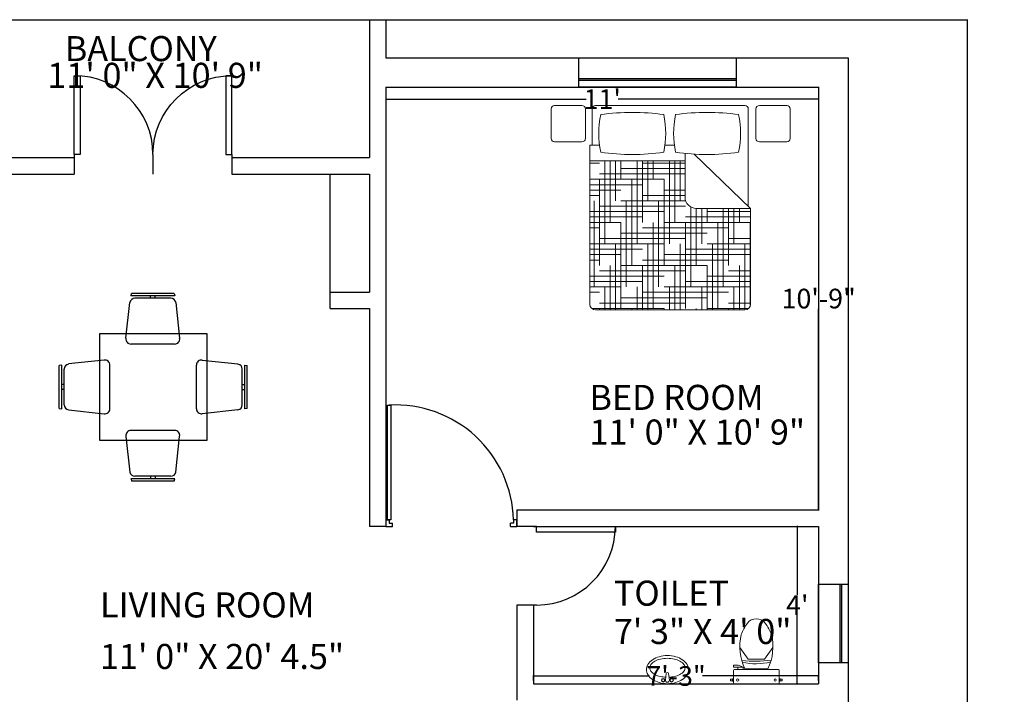
# Model space of a CAD drawing. Units: inches. Extents: x -113 to 5399, y -1393 to 3302.
# Tile 30 of 40: x 3870 to 4170, y 356 to 561. Entities that reach past the tile are written whole.
import ezdxf

# ---------------------------------------------------------------- set-up
doc = ezdxf.new("R2010")
doc.units = ezdxf.units.IN
doc.header["$MEASUREMENT"] = 0
for name, color, linetype, lineweight in [('A-ANNO-DIMS', 254, 'Continuous', 18), ('A-AREA-IDEN', 4, 'Continuous', 18), ('A-FLOR-FIXT', 8, 'Continuous', 18), ('doors', 2, 'Continuous', 25), ('furniture', 131, 'Continuous', 18), ('walls', 1, 'Continuous', 25), ('windows', 3, 'Continuous', 25)]:
    doc.layers.add(name, color=color, linetype=linetype, lineweight=lineweight)
doc.layers.add('B-FURNITURE', color=22, linetype='Continuous')
doc.styles.get("Standard").update_dxf_attribs({"font": 'arial.ttf'})
doc.dimstyles.get("Standard").update_dxf_attribs({"dimtxt": 6, "dimasz": 0.18, "dimexe": 0.18, "dimexo": 0.0625, "dimgap": 0.09, "dimtad": 0, "dimtih": 1, "dimtoh": 1, "dimdec": 1, "dimzin": 0, "dimdsep": 46, "dimlunit": 4, "dimtxsty": 'Standard', "dimblk": 'ARCHTICK', "dimcen": 0.09, "dimadec": 0, "dimazin": 0, "dimtfac": 1, "dimtdec": 1, "dimtofl": 0, "dimtmove": 0, "dimatfit": 3, "dimfxl": 1, "dimtolj": 1, "dimtzin": 0, "dimarcsym": 0})

# ---------------------------------------------------------------- blocks, each defined once
blk = doc.blocks.new('*U2')
for p, q in [((0, 0), (0, -6)), ((24, 0), (24, -6))]:
    blk.add_line(p, q)
blk.add_lwpolyline([(0, 0), (0, 24), (1.75, 24), (1.75, 0)], close=True)
blk.add_arc((0, 0), 24, 0, 90)
blk = doc.blocks.new('*X4')
at = {"color": 0}
for p, q in [((4.3594, 18.5625), (4.3594, 18.6457)), ((4.5, 18), (4.5, 18.6457)), ((4.5469, 18.1875), (4.5469, 18.6457)), ((4.5938, 18.375), (4.5938, 18.6457)), ((4.6406, 18.5625), (4.6406, 18.6457)), ((4.6875, 18.6094), (5.4375, 18.6094)), ((4.7812, 18), (4.7812, 18.6457)), ((4.8281, 18.1875), (4.8281, 18.6457)), ((4.875, 18.375), (4.875, 18.6457)), ((4.9219, 18.5625), (4.9219, 18.6457)), ((5.0625, 18), (5.0625, 18.6457)), ((5.1094, 18.1875), (5.1094, 18.6457)), ((5.1562, 18.375), (5.1562, 18.6457)), ((5.2031, 18.5625), (5.2031, 18.6457)), ((5.3438, 18), (5.3438, 18.6457)), ((5.3906, 18.1875), (5.3906, 18.6457)), ((5.4375, 18.375), (5.4375, 18.6457)), ((5.4844, 18.5625), (5.4844, 18.6457)), ((5.625, 18), (5.625, 18.6287)), ((4.4531, 17.8169), (4.4531, 18.5625)), ((4.5, 18.5625), (5.25, 18.5625)), ((4.7344, 17.8125), (4.7344, 18.5625)), ((5.0156, 17.8125), (5.0156, 18.5625)), ((5.2969, 17.8125), (5.2969, 18.5625)), ((5.5781, 17.8125), (5.5781, 18.5625)), ((5.625, 18.5625), (5.6375, 18.5625)), ((4.3395, 18.5156), (5.0625, 18.5156)), ((4.3395, 18.4688), (4.875, 18.4688)), ((5.25, 18.4688), (5.6375, 18.4688)), ((5.4375, 18.5156), (5.6375, 18.5156)), ((4.3395, 18.4219), (4.6875, 18.4219)), ((4.3395, 18.375), (4.5, 18.375)), ((4.4062, 17.8169), (4.4062, 18.375)), ((4.6875, 17.8114), (4.6875, 18.375)), ((4.875, 18.375), (5.625, 18.375)), ((4.9688, 17.625), (4.9688, 18.375)), ((5.0625, 18.4219), (5.6375, 18.4219)), ((5.25, 17.625), (5.25, 18.375)), ((5.5312, 17.625), (5.5312, 18.375)), ((4.5, 18.2812), (5.25, 18.2812)), ((4.6875, 18.3281), (5.4375, 18.3281)), ((5.625, 18.2812), (5.6375, 18.2812)), ((4.3395, 18.2344), (5.0625, 18.2344)), ((4.3395, 18.1875), (4.875, 18.1875)), ((4.3594, 17.8169), (4.3594, 18.1875)), ((4.6406, 17.8169), (4.6406, 18.1875)), ((4.9219, 17.4375), (4.9219, 18.1875)), ((5.2031, 17.4375), (5.2031, 18.1875)), ((5.25, 18.1875), (5.6375, 18.1875)), ((5.4375, 18.2344), (5.6375, 18.2344)), ((5.4844, 17.4375), (5.4844, 18.1875)), ((4.3395, 18.1406), (4.6875, 18.1406)), ((4.3395, 18.0938), (4.5, 18.0938)), ((4.875, 18.0938), (5.625, 18.0938)), ((5.0625, 18.1406), (5.6375, 18.1406)), ((4.6875, 18.0469), (5.4375, 18.0469)), ((4.3395, 17.9531), (5.0625, 17.9531)), ((4.5, 18), (5.25, 18)), ((4.5938, 17.8169), (4.5938, 18)), ((4.875, 17.25), (4.875, 18)), ((5.1562, 17.25), (5.1562, 18)), ((5.4375, 17.25), (5.4375, 18)), ((5.4375, 17.9531), (5.6375, 17.9531)), ((5.625, 18), (5.6375, 18)), ((4.3395, 17.9062), (4.875, 17.9062)), ((4.3395, 17.8594), (4.6875, 17.8594)), ((5.0625, 17.8594), (5.6375, 17.8594)), ((5.25, 17.9062), (5.6375, 17.9062)), ((4.7421, 17.7656), (5.4375, 17.7656)), ((4.8281, 17.2457), (4.8281, 17.8125)), ((4.875, 17.8125), (5.625, 17.8125)), ((5.1094, 17.2457), (5.1094, 17.8125)), ((5.3906, 17.2457), (5.3906, 17.8125)), ((4.7548, 17.7188), (5.25, 17.7188)), ((4.7548, 17.6719), (5.0625, 17.6719)), ((5.4375, 17.6719), (5.6375, 17.6719)), ((5.625, 17.7188), (5.6375, 17.7188)), ((4.7548, 17.625), (4.875, 17.625)), ((4.7812, 17.2457), (4.7812, 17.625)), ((5.0625, 17.2457), (5.0625, 17.625)), ((5.0625, 17.5781), (5.6375, 17.5781)), ((5.25, 17.625), (5.6375, 17.625)), ((5.3438, 17.2457), (5.3438, 17.625)), ((5.625, 17.2627), (5.625, 17.625)), ((4.875, 17.5312), (5.625, 17.5312)), ((4.7548, 17.4844), (5.4375, 17.4844)), ((4.7548, 17.4375), (5.25, 17.4375)), ((5.0156, 17.2457), (5.0156, 17.4375)), ((5.2969, 17.2457), (5.2969, 17.4375)), ((5.5781, 17.2457), (5.5781, 17.4375)), ((5.625, 17.4375), (5.6375, 17.4375)), ((4.7548, 17.3906), (5.0625, 17.3906)), ((4.7548, 17.3438), (4.875, 17.3438)), ((5.25, 17.3438), (5.6375, 17.3438)), ((5.4375, 17.3906), (5.6375, 17.3906)), ((4.875, 17.25), (5.6077, 17.25)), ((4.9688, 17.2457), (4.9688, 17.25)), ((5.0625, 17.2969), (5.6375, 17.2969)), ((5.25, 17.2457), (5.25, 17.25)), ((5.5312, 17.2457), (5.5312, 17.25))]:
    blk.add_line(p, q, dxfattribs=at)
blk = doc.blocks.new('MAT-P01')
for p, q in [((-0.0213, 0.8164), (-0.0213, 0.5605)), ((0.0087, 0.8464), (0.2471, 0.8464)), ((0.2771, 0.8164), (0.2771, 0.5605)), ((0.3437, 0.8164), (0.3437, -0.0316)), ((0.3737, 0.8464), (1.6737, 0.8464)), ((1.7037, 0.8164), (1.7037, 0.5005)), ((1.7622, 0.8164), (1.7622, 0.5605)), ((1.7922, 0.8464), (2.0306, 0.8464)), ((2.0606, 0.8164), (2.0606, 0.5605)), ((0.0087, 0.5305), (0.2471, 0.5305)), ((1.7922, 0.5305), (2.0306, 0.5305)), ((0.8949, 0.4293), (0.8949, 0.0491)), ((0.9879, 0.5005), (1.0693, 0.5005)), ((1.6393, 0.5005), (1.7237, 0.5005)), ((1.7237, 0.5005), (1.7237, -0.8836)), ((0.8146, 0.423), (0.3237, -0.0509)), ((0.8949, 0.3643), (1.7237, 0.3643)), ((0.8949, 0.3643), (0.8949, 0.0491)), ((0.8949, 0.3643), (1.7237, 0.3643)), ((1.7237, 0.3643), (1.7237, -0.8836)), ((0.3237, -0.0509), (0.7949, -0.0509)), ((0.3237, -0.0509), (0.3237, -0.8836)), ((0.3737, -0.9336), (1.6737, -0.9336))]:
    blk.add_line(p, q)
for centre, radius, start, end in [((0.0087, 0.8164), 0.03, 90, 180), ((0.2471, 0.8164), 0.03, 0, 90), ((0.3737, 0.8164), 0.03, 90, 180), ((0.7029, -1.1436), 1.9306, 81.81622, 98.18378), ((1.3543, -1.1436), 1.9306, 81.81622, 98.18378), ((1.6737, 0.8164), 0.03, 0, 90), ((1.7922, 0.8164), 0.03, 90, 180), ((2.0306, 0.8164), 0.03, 0, 90), ((1.2251, 0.6034), 0.8138, 168.37298, 191.62702), ((0.1806, 0.6034), 0.8138, 348.37298, 11.62702), ((1.8766, 0.6034), 0.8138, 168.37298, 191.62702), ((0.8321, 0.6034), 0.8138, 348.37298, 11.62702), ((0.0087, 0.5605), 0.03, 180, 270), ((0.2471, 0.5605), 0.03, 270, 0), ((1.7922, 0.5605), 0.03, 180, 270), ((2.0306, 0.5605), 0.03, 270, 0), ((0.7029, 2.3504), 1.9306, 261.81622, 278.18378), ((1.3543, 2.3504), 1.9306, 261.81622, 278.18378), ((0.7949, 0.0491), 0.1, 270, 0), ((0.3737, -0.8836), 0.05, 180, 270), ((1.6737, -0.8836), 0.05, 270, 0)]:
    blk.add_arc(centre, radius, start, end)
at = {"rotation": 270}
blk.add_blockref('*X4', (-16.9221, 4.7038), dxfattribs=at)
blk = doc.blocks.new('A$C6ACA79D1')
at = {"layer": 'B-FURNITURE'}
for p, q in [((-0.5034, 0.0535), (-0.8012, -0.2442)), ((-0.4835, 0.0392), (-0.7869, -0.2642)), ((-0.5034, 0.0535), (-0.4835, 0.0392)), ((-0.4291, 0.0003), (-0.1547, -0.2204)), ((0.7869, -0.259), (0.4835, 0.0444)), ((0.4842, 0.0434), (0.5041, 0.0577)), ((0.7427, -0.249), (0.4935, 0.0002)), ((0.8012, -0.239), (0.5034, 0.0587)), ((-0.4935, -0.005), (-0.7427, -0.2542)), ((-0.601, -0.1125), (-0.6181, -0.0954)), ((0.601, -0.1073), (0.6181, -0.0902)), ((-0.6352, -0.1467), (-0.6523, -0.1296)), ((0.6352, -0.1415), (0.6523, -0.1244)), ((-0.7859, -0.2635), (-0.8002, -0.2436)), ((0.8012, -0.239), (0.7869, -0.259)), ((-0.1485, -0.2964), (-0.4513, -0.5992)), ((0.4513, -0.594), (0.1485, -0.2912)), ((0.748, -0.3133), (0.5273, -0.5877)), ((-0.1485, -1.1937), (-0.4513, -0.8909)), ((0.4513, -0.8961), (0.1485, -1.199)), ((0.748, -1.1768), (0.5273, -0.9024)), ((-0.5034, -1.5436), (-0.8012, -1.2459)), ((-0.7859, -1.2266), (-0.8002, -1.2466)), ((-0.4835, -1.5293), (-0.7869, -1.226)), ((-0.4935, -1.4851), (-0.7427, -1.236)), ((0.7869, -1.2312), (0.4835, -1.5346)), ((0.7427, -1.2412), (0.4935, -1.4903)), ((0.8012, -1.2511), (0.5034, -1.5488)), ((0.8012, -1.2511), (0.7869, -1.2312)), ((-0.6352, -1.3434), (-0.6523, -1.3605)), ((-0.4291, -1.4904), (-0.1547, -1.2698)), ((0.6352, -1.3486), (0.6523, -1.3657)), ((-0.601, -1.3776), (-0.6181, -1.3948)), ((0.601, -1.3829), (0.6181, -1.4)), ((-0.5034, -1.5436), (-0.4835, -1.5293)), ((0.4842, -1.5336), (0.5041, -1.5478))]:
    blk.add_line(p, q, dxfattribs=at)
at = {"layer": 'B-FURNITURE', "ltscale": 300}
for p, q in [((0.1547, -0.2152), (0.4291, 0.0055)), ((-0.5273, -0.593), (-0.748, -0.3186)), ((-0.5273, -0.8972), (-0.748, -1.1716)), ((0.1547, -1.275), (0.4291, -1.4956))]:
    blk.add_line(p, q, dxfattribs=at)
blk.add_lwpolyline([(-0.7425, -0.7425), (0, 0), (0.7425, -0.7425), (0, -1.4849)], close=True, dxfattribs=at)
at = {"layer": 'B-FURNITURE', "ltscale": 400}
for centre, start, end in [((-0.4582, -0.0403), 54.40695, 135), ((0.4589, -0.0361), 45, 125.59305), ((-0.7063, -0.2888), 135, 215.59305), ((0.7073, -0.2843), 324.40695, 45), ((-0.7063, -1.2013), 144.40695, 225), ((0.7073, -1.2059), 315, 35.59305), ((-0.4582, -1.4498), 225, 305.59305), ((0.4589, -1.454), 234.40695, 315)]:
    blk.add_arc(centre, 0.0499, start, end, dxfattribs=at)
at = {"layer": 'B-FURNITURE', "ltscale": 300}
for centre, start, end in [((-0.1838, -0.261), 315, 54.40695), ((0.1838, -0.2558), 125.59305, 225), ((-0.4866, -0.5639), 215.59305, 315), ((0.4866, -0.5586), 225, 324.40695), ((-0.4866, -0.9263), 45, 144.40695), ((0.4866, -0.9315), 35.59305, 135), ((-0.1838, -1.2291), 305.59305, 45), ((0.1838, -1.2343), 135, 234.40695)]:
    blk.add_arc(centre, 0.05, start, end, dxfattribs=at)
blk = doc.blocks.new('toilet-3')
at = {"color": 0, "linetype": 'ByBlock'}
for p, q in [((-0.281, -0.05), (-0.281, -0.069)), ((-0.281, -0.05), (-0.261, -0.05)), ((-0.281, -0.069), (-0.261, -0.069)), ((-0.261, -0.047), (-0.261, -0.072)), ((-0.261, -0.047), (-0.251, -0.047)), ((-0.261, -0.072), (-0.251, -0.072)), ((-0.251, -0.047), (-0.251, -0.072)), ((-0.25, -0.03), (-0.25, -0.165)), ((0.24, -0.02), (-0.24, -0.02)), ((0.25, -0.03), (0.25, -0.165)), ((0.261, -0.047), (0.251, -0.047)), ((0.251, -0.047), (0.251, -0.072)), ((0.261, -0.072), (0.251, -0.072)), ((0.261, -0.047), (0.261, -0.072)), ((0.281, -0.05), (0.261, -0.05)), ((0.281, -0.069), (0.261, -0.069)), ((0.281, -0.05), (0.281, -0.069)), ((-0.144, -0.2), (-0.25, -0.2)), ((-0.25, -0.2), (-0.25, -0.222)), ((0.24, -0.175), (-0.24, -0.175)), ((-0.202, -0.2), (-0.202, -0.175)), ((-0.198, -0.222), (-0.16, -0.207)), ((-0.16, -0.207), (-0.16, -0.2)), ((-0.144, -0.2), (-0.144, -0.175)), ((0.125, -0.182), (-0.125, -0.182)), ((-0.198, -0.222), (-0.25, -0.222)), ((-0.089, -0.287), (-0.18, -0.415)), ((0.089, -0.287), (-0.089, -0.287)), ((0.089, -0.287), (0.18, -0.415))]:
    blk.add_line(p, q, dxfattribs=at)
for centre in [(-0.205, -0.059), (0.205, -0.059)]:
    blk.add_circle(centre, 0.0125, dxfattribs=at)
for centre, radius, start, end in [((-0.24, -0.03), 0.01, 90, 180), ((0.24, -0.03), 0.01, 0, 90), ((-0.24, -0.165), 0.01, 180, 270), ((0.376, -0.424), 0.557, 154.2321, 193.6755), ((-0.376, -0.424), 0.557, 346.3245, 25.7679), ((0.24, -0.165), 0.01, 270, 0), ((-0.013, -1.787), 1.521, 83.4552, 95.5271), ((-0.005, -0.896), 0.659, 75.9276, 103.0204), ((0.262, -0.406), 0.452, 199.2942, 217.2549), ((-0.265, -0.4), 0.457, 322.2382, 340.1051), ((-0.001, -0.609), 0.12, 216.3794, 323.6206)]:
    blk.add_arc(centre, radius, start, end, dxfattribs=at)
blk = doc.blocks.new('wash-6')
at = {"color": 0, "linetype": 'ByBlock'}
for p, q in [((-0.036, -0.063), (-0.021, -0.18)), ((0.036, -0.063), (0.021, -0.18))]:
    blk.add_line(p, q, dxfattribs=at)
for centre, radius in [((-0.075, -0.062), 0.0325), ((-0.075, -0.062), 0.0263), ((0.075, -0.062), 0.0325), ((0.075, -0.062), 0.0263)]:
    blk.add_circle(centre, radius, dxfattribs=at)
for centre, radius, start, end in [((0, -0.56), 0.56, 90, 105.4371), ((-0.204, -0.25), 0.17, 148.1465, 180), ((-0.107, -0.311), 0.285, 123.6901, 148.1465), ((-0.114, -0.361), 0.225, 118.369, 142.5096), ((-0.042, -0.407), 0.401, 105.4371, 123.6901), ((-0.045, -0.488), 0.37, 102.6081, 118.369), ((0, -0.69), 0.576, 92.9466, 102.6081), ((0, -0.063), 0.0361, 0, 180), ((0, -0.56), 0.56, 74.5629, 90), ((0, -0.69), 0.576, 77.3919, 87.0534), ((0.045, -0.488), 0.37, 61.631, 77.3919), ((0.042, -0.407), 0.401, 56.3099, 74.5629), ((0.114, -0.361), 0.225, 37.4904, 61.631), ((0.107, -0.311), 0.285, 31.8535, 56.3099), ((0.204, -0.25), 0.17, 0, 31.8535), ((-0.204, -0.25), 0.17, 180, 211.8535), ((-0.107, -0.189), 0.285, 211.8535, 236.3099), ((-0.217, -0.282), 0.0954, 142.5096, 180), ((-0.217, -0.282), 0.0954, 180, 217.4904), ((-0.114, -0.203), 0.225, 217.4904, 241.631), ((0, -0.18), 0.0215, 180, 0), ((0.114, -0.203), 0.225, 298.369, 322.5096), ((0.107, -0.189), 0.285, 303.6901, 328.1465), ((0.217, -0.282), 0.0954, 0, 37.4904), ((0.217, -0.282), 0.0954, 322.5096, 0), ((0.204, -0.25), 0.17, 328.1465, 0), ((-0.042, -0.092), 0.401, 236.3099, 254.5629), ((-0.045, -0.076), 0.37, 241.631, 257.3919), ((0, 0.06), 0.56, 254.5629, 270), ((0, 0.125), 0.576, 257.3919, 270), ((0, 0.125), 0.576, 270, 282.6081), ((0, 0.06), 0.56, 270, 285.4371), ((0.045, -0.076), 0.37, 282.6081, 298.369), ((0.042, -0.092), 0.401, 285.4371, 303.6901)]:
    blk.add_arc(centre, radius, start, end, dxfattribs=at)
blk = doc.blocks.new('_ArchTick')
at = {"color": 0, "linetype": 'ByBlock', "const_width": 0.15}
blk.add_lwpolyline([(-0.5, -0.5), (0.5, 0.5)], dxfattribs=at)
blk = doc.blocks.new('*D89')
at = {"layer": 'A-ANNO-DIMS', "color": 0, "lineweight": -2, "transparency": 16777216}
for p, q in [((4110.92, 540.78), (4113.91, 540.78)), ((4113.73, 540.78), (4113.73, 479.43)), ((4113.73, 411.78), (4113.73, 473.12)), ((4110.92, 411.78), (4113.91, 411.78))]:
    blk.add_line(p, q, dxfattribs=at)
at = {"layer": 'Defpoints', "color": 0, "transparency": 16777216}
for p in [(4110.86, 540.78), (4110.86, 411.78), (4113.73, 411.78)]:
    blk.add_point(p, dxfattribs=at)
at = {"layer": 'A-ANNO-DIMS', "color": 0, "lineweight": -2, "transparency": 16777216, "xscale": 0.18, "yscale": 0.18, "zscale": 0.18}
for p, rotation in [((4113.73, 540.78), 90), ((4113.73, 411.78), 270)]:
    blk.add_blockref('_ArchTick', p, dxfattribs=dict(at, rotation=rotation))
at = {"layer": 'A-ANNO-DIMS', "color": 0, "transparency": 16777216, "insert": (4113.73, 476.28), "char_height": 6, "attachment_point": 5}
blk.add_mtext('\\A1;10\'-9"', dxfattribs=at)
blk = doc.blocks.new('*D90')
at = {"layer": 'A-ANNO-DIMS', "color": 0, "lineweight": -2, "transparency": 16777216}
for p, q in [((3981.73, 537.14), (4042.83, 537.14)), ((3981.73, 537.08), (3981.73, 536.96)), ((4113.73, 537.14), (4052.63, 537.14)), ((4113.73, 537.2), (4113.73, 537.32))]:
    blk.add_line(p, q, dxfattribs=at)
at = {"layer": 'Defpoints', "color": 0, "transparency": 16777216}
for p in [(3981.73, 537.14), (4113.73, 537.14), (4113.73, 537.14)]:
    blk.add_point(p, dxfattribs=at)
at = {"layer": 'A-ANNO-DIMS', "color": 0, "lineweight": -2, "transparency": 16777216, "xscale": 0.18, "yscale": 0.18, "zscale": 0.18, "rotation": 180}
blk.add_blockref('_ArchTick', (3981.73, 537.14), dxfattribs=at)
at = {"layer": 'A-ANNO-DIMS', "color": 0, "lineweight": -2, "transparency": 16777216, "xscale": 0.18, "yscale": 0.18, "zscale": 0.18}
blk.add_blockref('_ArchTick', (4113.73, 537.14), dxfattribs=at)
at = {"layer": 'A-ANNO-DIMS', "color": 0, "transparency": 16777216, "insert": (4047.73, 537.14), "char_height": 6, "attachment_point": 5}
blk.add_mtext("\\A1;11'", dxfattribs=at)
blk = doc.blocks.new('*D91')
at = {"layer": 'A-ANNO-DIMS', "color": 0, "lineweight": -2, "transparency": 16777216}
for p, q in [((4107.38, 406.78), (4107.03, 406.78)), ((4107.21, 406.78), (4107.21, 385.87)), ((4107.21, 358.78), (4107.21, 379.69)), ((4107.38, 358.78), (4107.03, 358.78))]:
    blk.add_line(p, q, dxfattribs=at)
at = {"layer": 'Defpoints', "color": 0, "transparency": 16777216}
for p in [(4107.45, 406.78), (4107.21, 358.78), (4107.45, 358.78)]:
    blk.add_point(p, dxfattribs=at)
at = {"layer": 'A-ANNO-DIMS', "color": 0, "lineweight": -2, "transparency": 16777216, "xscale": 0.18, "yscale": 0.18, "zscale": 0.18}
for p, rotation in [((4107.21, 406.78), 90), ((4107.21, 358.78), 270)]:
    blk.add_blockref('_ArchTick', p, dxfattribs=dict(at, rotation=rotation))
at = {"layer": 'A-ANNO-DIMS', "color": 0, "transparency": 16777216, "insert": (4107.21, 382.78), "char_height": 6, "attachment_point": 5}
blk.add_mtext("\\A1;4'", dxfattribs=at)
blk = doc.blocks.new('*D94')
at = {"layer": 'A-ANNO-DIMS', "color": 0, "lineweight": -2, "transparency": 16777216}
for p, q in [((4026.73, 359.8), (4026.73, 361.31)), ((4026.73, 361.13), (4062.19, 361.13)), ((4113.73, 361.13), (4078.27, 361.13)), ((4113.73, 359.8), (4113.73, 361.31))]:
    blk.add_line(p, q, dxfattribs=at)
at = {"layer": 'Defpoints', "color": 0, "transparency": 16777216}
for p in [(4026.73, 361.13), (4026.73, 359.73), (4113.73, 359.73)]:
    blk.add_point(p, dxfattribs=at)
at = {"layer": 'A-ANNO-DIMS', "color": 0, "lineweight": -2, "transparency": 16777216, "xscale": 0.18, "yscale": 0.18, "zscale": 0.18, "rotation": 180}
blk.add_blockref('_ArchTick', (4026.73, 361.13), dxfattribs=at)
at = {"layer": 'A-ANNO-DIMS', "color": 0, "lineweight": -2, "transparency": 16777216, "xscale": 0.18, "yscale": 0.18, "zscale": 0.18}
blk.add_blockref('_ArchTick', (4113.73, 361.13), dxfattribs=at)
at = {"layer": 'A-ANNO-DIMS', "color": 0, "transparency": 16777216, "insert": (4070.23, 361.13), "char_height": 6, "attachment_point": 5}
blk.add_mtext('\\A1;7\'-3"', dxfattribs=at)
blk = doc.blocks.new('WIN-PLAN-48IN')
h = blk.add_hatch(color=256)
h.dxf.hatch_style = 1
h.paths.add_polyline_path([(48, 2.5), (0, 2.5), (0, 2), (48, 2)])
for p, q in [((0, 9), (48, 9)), ((0, 0), (0, 9)), ((48, 9), (48, 0)), ((48, 2.5), (0, 2.5)), ((48, 2), (0, 2)), ((48, 0), (0, 0))]:
    blk.add_line(p, q)
blk = doc.blocks.new('WIN-PLAN-24IN')
h = blk.add_hatch(color=256)
h.dxf.hatch_style = 1
h.paths.add_polyline_path([(6.5, 24), (6.5, 0), (7, 0), (7, 24)])
for p, q in [((0, 0), (0, 24)), ((0, 24), (9, 24)), ((6.5, 24), (6.5, 0)), ((7, 24), (7, 0)), ((9, 24), (9, 0)), ((9, 0), (0, 0))]:
    blk.add_line(p, q)
blk = doc.blocks.new('DOOR-SINGLE-36IN-PLAN')
for p, q in [((0.5, 2), (0.5, 36.98)), ((0.5, 36.98), (1.5, 36.98)), ((1.5, 36.98), (1.5, 2)), ((0, 2), (0, 0)), ((0, 2), (1.04, 2)), ((1.5, 2), (0.5, 2)), ((1.04, 2), (1.04, 0.98)), ((1.04, 0.98), (2, 0.98)), ((2, 0), (2, 0.98)), ((38.96, 0.98), (38, 0.98)), ((38, 0), (38, 0.98)), ((40, 2), (38.96, 2)), ((38.96, 2), (38.96, 0.98)), ((40, 0), (40, 2)), ((0, 0), (2, 0)), ((0, 0), (2, 0)), ((38, 0), (40, 0))]:
    blk.add_line(p, q)
blk.add_arc((2.94, 0.99), 36.04, 1.6003, 93.0893)
blk = doc.blocks.new('*D185')
at = {"layer": 'A-ANNO-DIMS', "color": 0, "lineweight": -2, "transparency": 16777216}
for p, q in [((3889.72, 345.5), (3889.54, 345.5)), ((3889.72, 332.93), (3889.72, 345.68)), ((3973.94, 345.5), (3889.72, 345.5)), ((3973.94, 332.93), (3973.94, 345.68))]:
    blk.add_line(p, q, dxfattribs=at)
at = {"layer": 'Defpoints', "color": 0, "transparency": 16777216}
for p in [(3889.72, 345.5), (3889.72, 332.87), (3973.94, 332.87)]:
    blk.add_point(p, dxfattribs=at)
at = {"layer": 'A-ANNO-DIMS', "color": 0, "lineweight": -2, "transparency": 16777216, "xscale": 0.18, "yscale": 0.18, "zscale": 0.18, "rotation": 180}
blk.add_blockref('_ArchTick', (3889.72, 345.5), dxfattribs=at)
at = {"layer": 'A-ANNO-DIMS', "color": 0, "lineweight": -2, "transparency": 16777216, "xscale": 0.18, "yscale": 0.18, "zscale": 0.18}
blk.add_blockref('_ArchTick', (3973.94, 345.5), dxfattribs=at)
at = {"layer": 'A-ANNO-DIMS', "color": 0, "transparency": 16777216, "insert": (3835.08, 345.5), "char_height": 6, "attachment_point": 5}
blk.add_mtext('\\A1;SEATING GROUP 7\'-0" TYP.', dxfattribs=at)
blk = doc.blocks.new('*D210')
at = {"layer": 'A-ANNO-DIMS', "color": 0, "lineweight": -2, "transparency": 16777216}
for p, q in [((3839.79, 561.28), (4159.21, 561.28)), ((4159.03, 561.28), (4159.03, 230.43)), ((4159.03, -106.72), (4159.03, 224.12)), ((3839.79, -106.72), (4159.21, -106.72))]:
    blk.add_line(p, q, dxfattribs=at)
at = {"layer": 'Defpoints', "color": 0, "transparency": 16777216}
for p in [(3839.73, 561.28), (4159.03, 561.28), (3839.73, -106.72)]:
    blk.add_point(p, dxfattribs=at)
at = {"layer": 'A-ANNO-DIMS', "color": 0, "lineweight": -2, "transparency": 16777216, "xscale": 0.18, "yscale": 0.18, "zscale": 0.18}
for p, rotation in [((4159.03, 561.28), 90), ((4159.03, -106.72), 270)]:
    blk.add_blockref('_ArchTick', p, dxfattribs=dict(at, rotation=rotation))
at = {"layer": 'A-ANNO-DIMS', "color": 0, "transparency": 16777216, "insert": (4159.03, 227.28), "char_height": 6, "attachment_point": 5}
blk.add_mtext('\\A1;55\'-8"', dxfattribs=at)

msp = doc.modelspace()

# ---------------------------------------------------------------- linework, layer by layer
at = {"layer": 'walls'}
for p, q in [((3844.73, 561.28), (3976.73, 561.28)), ((3976.73, 561.28), (3976.73, 519.28)), ((3976.73, 561.28), (3981.73, 561.28)), ((3981.73, 561.28), (3981.73, 549.78)), ((3981.73, 549.78), (4122.73, 549.78)), ((4122.73, 549.78), (4122.73, -100.22)), ((3981.73, 540.78), (3981.73, 406.78)), ((3981.73, 540.78), (4113.73, 540.78)), ((4113.73, 540.78), (4113.73, 411.78)), ((3844.73, 519.28), (3886.73, 519.28)), ((3886.73, 519.28), (3886.73, 514.28)), ((3934.73, 519.28), (3976.73, 519.28)), ((3934.73, 519.28), (3934.73, 514.28)), ((3844.73, 514.28), (3886.73, 514.28)), ((3934.73, 514.28), (3976.73, 514.28)), ((3964.73, 478.28), (3964.73, 514.28)), ((3976.73, 514.28), (3976.73, 478.28)), ((3964.73, 478.28), (3976.73, 478.28)), ((3964.73, 473.28), (3964.73, 478.28)), ((3964.73, 473.28), (3976.73, 473.28)), ((3976.73, 473.28), (3976.73, 406.78)), ((4021.73, 411.78), (4021.73, 406.78)), ((4021.73, 411.78), (4113.73, 411.78)), ((3981.73, 406.78), (3976.73, 406.78)), ((4026.73, 406.78), (4021.73, 406.78)), ((4026.73, 406.78), (4113.73, 406.78)), ((4113.73, 406.78), (4113.73, 358.78)), ((4021.73, 382.78), (4021.73, 353.78)), ((4026.73, 382.78), (4021.73, 382.78)), ((4026.73, 382.78), (4026.73, 358.78)), ((4026.73, 358.78), (4113.73, 358.78))]:
    msp.add_line(p, q, dxfattribs=at)

# ---------------------------------------------------------------- block references
at = {"layer": 'A-FLOR-FIXT', "rotation": 180}
for name, p, xscale, yscale, zscale in [('toilet-3', (4094.73, 358.22), -27.95492935005888, 27.95492935005888, 27.95492935005888), ('wash-6', (4067.61, 358.78), -17.16666334294967, 17.16666334294967, 17.16666334294967)]:
    msp.add_blockref(name, p, dxfattribs=dict(at, xscale=xscale, yscale=yscale, zscale=zscale))
at = {"layer": 'doors'}
for name, p in [('*U2', (3886.73, 520.28)), ('DOOR-SINGLE-36IN-PLAN', (3981.73, 406.78))]:
    msp.add_blockref(name, p, dxfattribs=at)
at = {"layer": 'doors', "xscale": -1}
msp.add_blockref('*U2', (3934.73, 520.28), dxfattribs=at)
at = {"layer": 'doors', "rotation": 270}
msp.add_blockref('*U2', (4027.73, 406.78), dxfattribs=at)
at = {"layer": 'furniture', "xscale": -35.02364872074636, "yscale": 35.02364872074636, "zscale": 35.02364872074636}
msp.add_blockref('MAT-P01', (4104.32, 505.53), dxfattribs=at)
at = {"layer": 'furniture', "xscale": 31.0665876167328, "yscale": 31.0665876167328, "zscale": 31.0665876167328, "rotation": 314.9999999999397}
msp.add_blockref('A$C6ACA79D1', (3927.11, 465.64), dxfattribs=at)
at = {"layer": 'windows'}
for name, p in [('WIN-PLAN-48IN', (4040.55, 540.78)), ('WIN-PLAN-24IN', (4113.73, 365.15))]:
    msp.add_blockref(name, p, dxfattribs=at)

# ---------------------------------------------------------------- texts
at = {"layer": 'A-AREA-IDEN'}
for s, height, p in [('BALCONY', 7.647, (3883.85, 548.73)), ('11\' 0" X 10\' 9"', 7.6473, (3878.52, 540.57)), ('BED ROOM', 7.647, (4043.84, 442.31)), ('11\' 0" X 10\' 9"', 7.6473, (4043.84, 431.73)), ('TOILET', 7.647, (4051.27, 382.57)), ('LIVING ROOM', 7.6473, (3894.58, 378.98)), ('7\' 3" X 4\' 0"', 7.6473, (4051.27, 370.89)), ('11\' 0" X 20\' 4.5"', 7.6473, (3894.58, 363.26))]:
    msp.add_text(s, height=height, dxfattribs=at).set_placement(p)

# ---------------------------------------------------------------- dimensions: what is measured, and where the dimension line sits
at = {"layer": 'A-ANNO-DIMS'}
for base, p1, p2, override, picture, middle in [((4159.03, 561.28), (3839.73, -106.72), (3839.73, 561.28), {"dimdec": 1, "dimlfac": 1, "dimrnd": 0, "dimzin": 1, "dimdsep": 46, "dimlunit": 4, "dimfrac": 2}, '*D210', (4159.03, 227.28)), ((4113.73, 411.78), (4110.86, 540.78), (4110.86, 411.78), {"dimclrd": 0, "dimclre": 0, "dimclrt": 0}, '*D89', (4113.73, 476.28)), ((4107.21, 358.78), (4107.45, 406.78), (4107.45, 358.78), {"dimclrd": 0, "dimclre": 0, "dimclrt": 0}, '*D91', (4107.21, 382.78))]:
    dim = msp.add_linear_dim(base=base, p1=p1, p2=p2, angle=90, dimstyle='Standard', override=override, dxfattribs=at)
    dim.commit()
    dim.dimension.update_dxf_attribs({"geometry": picture, "text_midpoint": middle})
for base, p1, p2, picture, middle in [((4113.73, 537.14), (3981.73, 537.14), (4113.73, 537.14), '*D90', (4047.73, 537.14)), ((4026.73, 361.13), (4113.73, 359.73), (4026.73, 359.73), '*D94', (4070.23, 361.13))]:
    dim = msp.add_linear_dim(base=base, p1=p1, p2=p2, dimstyle='Standard', override={"dimclrd": 0, "dimclre": 0, "dimclrt": 0}, dxfattribs=at)
    dim.commit()
    dim.dimension.update_dxf_attribs({"geometry": picture, "text_midpoint": middle})
dim = msp.add_linear_dim(base=(3889.72, 345.5), p1=(3973.94, 332.87), p2=(3889.72, 332.87), angle=180, text='SEATING GROUP <> TYP.', dimstyle='Standard', override={"dimdec": 1, "dimlfac": 1, "dimrnd": 0, "dimzin": 1, "dimdsep": 46, "dimlunit": 4, "dimfrac": 2}, dxfattribs=at)
dim.commit()
dim.dimension.update_dxf_attribs({"geometry": '*D185', "text_midpoint": (3835.08, 345.5)})

doc.saveas('drawing.dxf')
